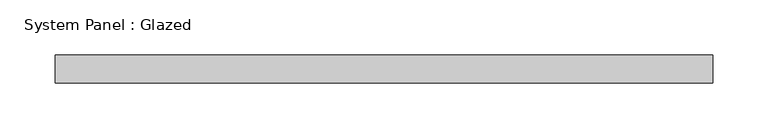
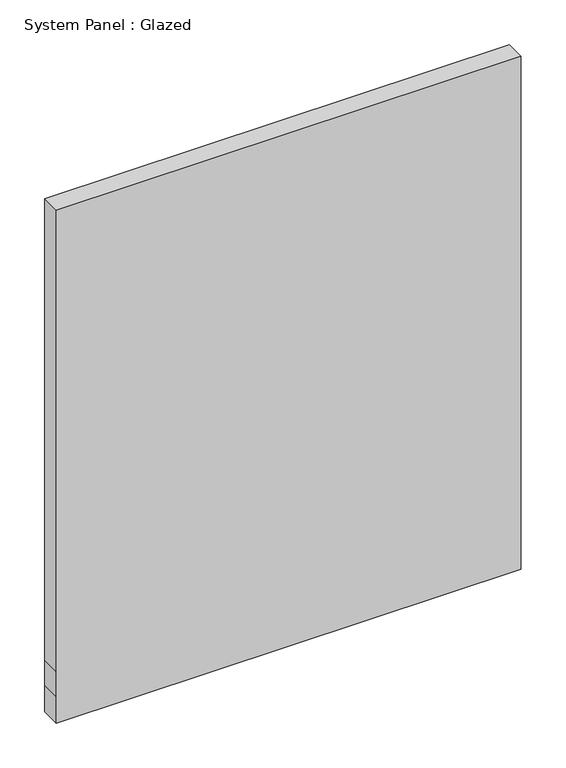
"""IFC4 building model written with IfcOpenShell, lengths in millimetres: plate geometry, System Panel : Glazed."""

from ifc_helpers import new_model, si_unit, frame, origin, place, context, project, spatial, polyline, outline, extrude, source, transform, mapped, element, save


def system_panel_glazed_000d40f8(model_context):
    return source(origin(), model_context, "Body", "SweptSolid", [
        extrude(outline(polyline([(0.0, -298.45), (0.0, 298.45), (35.9833333, 298.45), (69.85, 298.45), (696.0441631, 298.45), (696.0441631, -298.45), (69.85, -298.45), (35.9833333, -298.45), (0.0, -298.45)])), frame((0.0, 19.05, 0.0), z_axis=(0.0, 1.0, 0.0), x_axis=(0.0, 0.0, 1.0)), (0.0, 0.0, 1.0), 25.4),
    ])


if __name__ == "__main__":
    model = new_model("IFC4")
    model_context = context("Model", 3, world=origin())
    ifc_project = project(units=[si_unit("LENGTHUNIT", "METRE", prefix="MILLI")], contexts=[model_context])
    site = spatial("IfcSite", under=ifc_project)
    building = spatial("IfcBuilding", under=site)
    placement = place(None, origin())
    system_panel_glazed_shape = system_panel_glazed_000d40f8(model_context)
    element("IfcPlate", 1, ObjectType="System Panel : Glazed", at=placement, inside=building, context=model_context, shape_type="MappedRepresentation", body=[
        mapped(system_panel_glazed_shape, transform((0.0, 0.0, 0.0), x_axis=(1.0, 0.0, 0.0), y_axis=(0.0, 1.0, 0.0), z_axis=(0.0, 0.0, 1.0))),
    ])
    save(model, "model.ifc")

# Revit data of these elements
# Type "System Panel : Glazed"
#   Construction Type Id = "GSP4R"
#   Analytic Construction = "1/8 in Pilkington single glazing"
#   Visual Light Transmittance = 0.9
#   Solar Heat Gain Coefficient = 0.86
#   Heat Transfer Coefficient (U) = 1.18115 BTU/(h·ft²·°F)
#   Define Thermal Properties by = 1
# Element 1 (IfcPlate, "System Panel : Glazed")
#   Materials on its faces: "Glass"
# Materials
#   "Glass": class "Glass", colour RGB 0 128 192, transparency 0.75, Description = "Soda Lime Glass", Cost = 0
